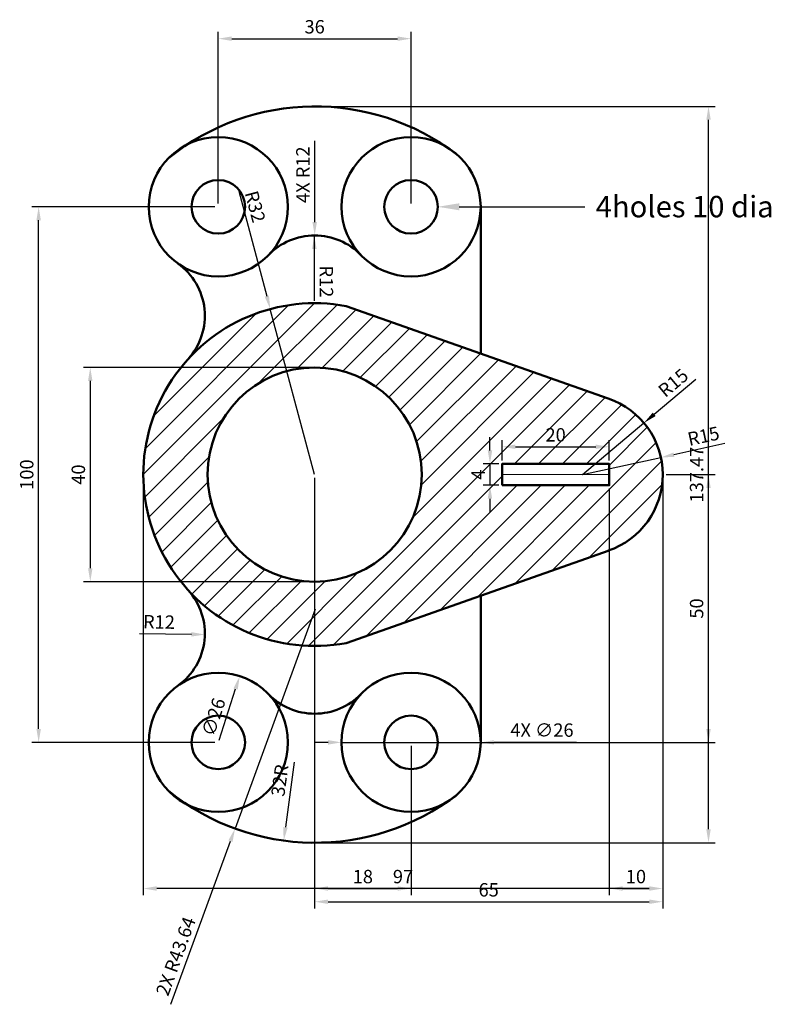
# Model space of a CAD drawing. Units: millimetres. Extents: x 3469 to 3609, y 1274 to 1457.
import ezdxf
from ezdxf import colors
from ezdxf.entities.mleader import LeaderData, LeaderLine
from ezdxf.math import Vec2, Vec3

# ---------------------------------------------------------------- set-up
doc = ezdxf.new("R2010")
doc.units = ezdxf.units.MM
doc.linetypes.add('CENTER', pattern=[50.8, 31.75, -6.35, 6.35, -6.35])
for name, color, linetype, lineweight in [('M-CNTR', 4, 'CENTER', 18), ('M-DIMS', 2, 'Continuous', 25), ('M-HATC', 8, 'Continuous', 18), ('M-OUTL', 7, 'Continuous', 50), ('M-TEXT', 7, 'Continuous', 25)]:
    doc.layers.add(name, color=color, linetype=linetype, lineweight=lineweight)
doc.styles.get("Standard").update_dxf_attribs({"font": 'arial.ttf'})
doc.dimstyles.new('ISO-25', dxfattribs={"dimtxt": 2.5, "dimasz": 2.5, "dimexe": 1.25, "dimexo": 0.625, "dimtad": 1, "dimtxsty": 'Standard', "dimcen": 2.5, "dimadec": 0, "dimazin": 0, "dimtfac": 1, "dimtmove": 0, "dimatfit": 3, "dimfxl": 1, "dimarcsym": 0})

# ---------------------------------------------------------------- blocks, each defined once
blk = doc.blocks.new('*D1')
at = {"layer": 'Defpoints', "color": 0, "transparency": 16777216}
for p in [(3541.88, 1453.9), (3505.88, 1422.51), (3541.88, 1422.51)]:
    blk.add_point(p, dxfattribs=at)
at = {"layer": 'M-DIMS', "color": 0, "lineweight": -2, "transparency": 16777216}
for p, q in [((3505.88, 1423.14), (3505.88, 1455.15)), ((3541.88, 1423.14), (3541.88, 1455.15)), ((3508.38, 1453.9), (3539.38, 1453.9))]:
    blk.add_line(p, q, dxfattribs=at)
at = {"layer": 'M-DIMS', "color": 0, "transparency": 16777216}
for points in [[(3508.38, 1454.32), (3508.38, 1453.49), (3505.88, 1453.9)], [(3539.38, 1454.32), (3539.38, 1453.49), (3541.88, 1453.9)]]:
    blk.add_solid(points, dxfattribs=at)
at = {"layer": 'M-DIMS', "color": 0, "transparency": 16777216, "insert": (3523.88, 1455.8), "char_height": 2.5, "attachment_point": 5}
blk.add_mtext('36', dxfattribs=at)
blk = doc.blocks.new('*D2')
at = {"layer": 'Defpoints', "color": 0, "transparency": 16777216}
for p in [(3523.88, 1372.51), (3588.88, 1372.51), (3588.88, 1292.76)]:
    blk.add_point(p, dxfattribs=at)
at = {"layer": 'M-DIMS', "color": 0, "lineweight": -2, "transparency": 16777216}
for p, q in [((3523.88, 1371.89), (3523.88, 1291.51)), ((3588.88, 1371.89), (3588.88, 1291.51)), ((3526.38, 1292.76), (3586.38, 1292.76))]:
    blk.add_line(p, q, dxfattribs=at)
at = {"layer": 'M-DIMS', "color": 0, "transparency": 16777216}
for points in [[(3526.38, 1293.17), (3526.38, 1292.34), (3523.88, 1292.76)], [(3586.38, 1293.17), (3586.38, 1292.34), (3588.88, 1292.76)]]:
    blk.add_solid(points, dxfattribs=at)
at = {"layer": 'M-DIMS', "color": 0, "transparency": 16777216, "insert": (3556.38, 1294.66), "char_height": 2.5, "attachment_point": 5}
blk.add_mtext('65', dxfattribs=at)
blk = doc.blocks.new('*D3')
at = {"layer": 'Defpoints', "color": 0, "transparency": 16777216}
for p in [(3472.33, 1422.51), (3505.88, 1422.51), (3505.88, 1322.51)]:
    blk.add_point(p, dxfattribs=at)
at = {"layer": 'M-DIMS', "color": 0, "lineweight": -2, "transparency": 16777216}
for p, q in [((3505.26, 1422.51), (3471.08, 1422.51)), ((3472.33, 1325.01), (3472.33, 1420.01)), ((3505.26, 1322.51), (3471.08, 1322.51))]:
    blk.add_line(p, q, dxfattribs=at)
at = {"layer": 'M-DIMS', "color": 0, "transparency": 16777216}
for points in [[(3471.92, 1420.01), (3472.75, 1420.01), (3472.33, 1422.51)], [(3471.92, 1325.01), (3472.75, 1325.01), (3472.33, 1322.51)]]:
    blk.add_solid(points, dxfattribs=at)
at = {"layer": 'M-DIMS', "color": 0, "transparency": 16777216, "insert": (3470.43, 1372.51), "char_height": 2.5, "attachment_point": 5, "rotation": 90}
blk.add_mtext('100', dxfattribs=at)
blk = doc.blocks.new('*D4')
at = {"layer": 'Defpoints', "color": 0, "transparency": 16777216}
for p in [(3523.88, 1392.51), (3481.97, 1352.51), (3523.88, 1352.51)]:
    blk.add_point(p, dxfattribs=at)
at = {"layer": 'M-DIMS', "color": 0, "lineweight": -2, "transparency": 16777216}
for p, q in [((3523.26, 1392.51), (3480.72, 1392.51)), ((3481.97, 1390.01), (3481.97, 1355.01)), ((3523.26, 1352.51), (3480.72, 1352.51))]:
    blk.add_line(p, q, dxfattribs=at)
at = {"layer": 'M-DIMS', "color": 0, "transparency": 16777216}
for points in [[(3481.56, 1390.01), (3482.39, 1390.01), (3481.97, 1392.51)], [(3481.56, 1355.01), (3482.39, 1355.01), (3481.97, 1352.51)]]:
    blk.add_solid(points, dxfattribs=at)
at = {"layer": 'M-DIMS', "color": 0, "transparency": 16777216, "insert": (3480.07, 1372.51), "char_height": 2.5, "attachment_point": 5, "rotation": 90}
blk.add_mtext('40', dxfattribs=at)
blk = doc.blocks.new('*D5')
at = {"layer": 'Defpoints', "color": 0, "transparency": 16777216}
for p in [(3578.88, 1377.7), (3558.88, 1374.51), (3578.88, 1374.51)]:
    blk.add_point(p, dxfattribs=at)
at = {"layer": 'M-DIMS', "color": 0, "lineweight": -2, "transparency": 16777216}
for p, q in [((3558.88, 1375.14), (3558.88, 1378.95)), ((3578.88, 1375.14), (3578.88, 1378.95)), ((3561.38, 1377.7), (3576.38, 1377.7))]:
    blk.add_line(p, q, dxfattribs=at)
at = {"layer": 'M-DIMS', "color": 0, "transparency": 16777216}
for points in [[(3561.38, 1378.12), (3561.38, 1377.29), (3558.88, 1377.7)], [(3576.38, 1378.12), (3576.38, 1377.29), (3578.88, 1377.7)]]:
    blk.add_solid(points, dxfattribs=at)
at = {"layer": 'M-DIMS', "color": 0, "transparency": 16777216, "insert": (3568.88, 1379.61), "char_height": 2.5, "attachment_point": 5}
blk.add_mtext('20', dxfattribs=at)
blk = doc.blocks.new('*D6')
at = {"layer": 'Defpoints', "color": 0, "transparency": 16777216}
for p in [(3558.88, 1374.51), (3556.62, 1370.51), (3558.88, 1370.51)]:
    blk.add_point(p, dxfattribs=at)
at = {"layer": 'M-DIMS', "color": 0, "lineweight": -2, "transparency": 16777216}
for p, q in [((3556.62, 1377.01), (3556.62, 1379.51)), ((3558.26, 1374.51), (3555.37, 1374.51)), ((3556.62, 1374.51), (3556.62, 1370.51)), ((3558.26, 1370.51), (3555.37, 1370.51)), ((3556.62, 1368.01), (3556.62, 1365.51))]:
    blk.add_line(p, q, dxfattribs=at)
at = {"layer": 'M-DIMS', "color": 0, "transparency": 16777216}
for points in [[(3556.2, 1377.01), (3557.03, 1377.01), (3556.62, 1374.51)], [(3556.2, 1368.01), (3557.03, 1368.01), (3556.62, 1370.51)]]:
    blk.add_solid(points, dxfattribs=at)
at = {"layer": 'M-DIMS', "color": 0, "transparency": 16777216, "insert": (3554.74, 1372.51), "char_height": 2.5, "attachment_point": 5, "rotation": 90}
blk.add_mtext('4', dxfattribs=at)
blk = doc.blocks.new('*D7')
at = {"layer": 'Defpoints', "color": 0, "transparency": 16777216}
for p in [(3509.89, 1334.88), (3501.88, 1310.14)]:
    blk.add_point(p, dxfattribs=at)
at = {"layer": 'M-DIMS', "color": 0, "lineweight": -2, "transparency": 16777216}
blk.add_line((3506.02, 1322.94), (3509.12, 1332.5), dxfattribs=at)
at = {"layer": 'M-DIMS', "color": 0, "transparency": 16777216}
blk.add_solid([(3508.72, 1332.63), (3509.51, 1332.37), (3509.89, 1334.88)], dxfattribs=at)
at = {"layer": 'M-DIMS', "color": 0, "transparency": 16777216, "insert": (3505.31, 1327.14), "char_height": 2.5, "attachment_point": 5, "rotation": 72.0514}
blk.add_mtext('∅26', dxfattribs=at)
blk = doc.blocks.new('*D8')
at = {"layer": 'Defpoints', "color": 0, "transparency": 16777216}
for p in [(3523.96, 1347.41), (3518.09, 1304.17)]:
    blk.add_point(p, dxfattribs=at)
at = {"layer": 'M-DIMS', "color": 0, "lineweight": -2, "transparency": 16777216}
blk.add_line((3520.08, 1318.8), (3518.43, 1306.65), dxfattribs=at)
at = {"layer": 'M-DIMS', "color": 0, "transparency": 16777216}
blk.add_solid([(3518.01, 1306.7), (3518.84, 1306.59), (3518.09, 1304.17)], dxfattribs=at)
at = {"layer": 'M-DIMS', "color": 0, "transparency": 16777216, "insert": (3517.69, 1315.36), "char_height": 2.5, "attachment_point": 5, "rotation": 82.2703}
blk.add_mtext('32R', dxfattribs=at)
blk = doc.blocks.new('*D9')
at = {"layer": 'Defpoints', "color": 0, "transparency": 16777216}
for p in [(3588.54, 1375.7), (3573.88, 1372.51)]:
    blk.add_point(p, dxfattribs=at)
at = {"layer": 'M-DIMS', "color": 0, "lineweight": -2, "transparency": 16777216}
for p, q in [((3600.5, 1378.3), (3590.98, 1376.23)), ((3573.88, 1372.51), (3588.54, 1375.7))]:
    blk.add_line(p, q, dxfattribs=at)
at = {"layer": 'M-DIMS', "color": 0, "transparency": 16777216}
blk.add_solid([(3590.89, 1376.64), (3591.07, 1375.82), (3588.54, 1375.7)], dxfattribs=at)
at = {"layer": 'M-DIMS', "color": 0, "transparency": 16777216, "insert": (3596.56, 1379.39), "char_height": 2.5, "attachment_point": 5, "rotation": 12.2647}
blk.add_mtext('R15', dxfattribs=at)
blk = doc.blocks.new('*D10')
at = {"layer": 'Defpoints', "color": 0, "transparency": 16777216}
for p in [(3491.37, 1342.87), (3503.37, 1342.64)]:
    blk.add_point(p, dxfattribs=at)
at = {"layer": 'M-DIMS', "color": 0, "lineweight": -2, "transparency": 16777216}
blk.add_line((3491.17, 1342.87), (3500.87, 1342.69), dxfattribs=at)
at = {"layer": 'M-DIMS', "color": 0, "transparency": 16777216}
blk.add_solid([(3500.87, 1343.1), (3500.86, 1342.27), (3503.37, 1342.64)], dxfattribs=at)
at = {"layer": 'M-DIMS', "color": 0, "transparency": 16777216, "insert": (3494.8, 1344.68), "char_height": 2.5, "attachment_point": 5, "rotation": 358.9032}
blk.add_mtext('R12', dxfattribs=at)
blk = doc.blocks.new('*D11')
at = {"layer": 'Defpoints', "color": 0, "transparency": 16777216}
for p in [(3523.81, 1417.16), (3523.88, 1405.16)]:
    blk.add_point(p, dxfattribs=at)
at = {"layer": 'M-DIMS', "color": 0, "lineweight": -2, "transparency": 16777216}
blk.add_line((3523.88, 1404.96), (3523.83, 1414.66), dxfattribs=at)
at = {"layer": 'M-DIMS', "color": 0, "transparency": 16777216}
blk.add_solid([(3524.24, 1414.66), (3523.41, 1414.66), (3523.81, 1417.16)], dxfattribs=at)
at = {"layer": 'M-DIMS', "color": 0, "transparency": 16777216, "insert": (3525.74, 1408.57), "char_height": 2.5, "attachment_point": 5, "rotation": 270.331}
blk.add_mtext('R12', dxfattribs=at)
blk = doc.blocks.new('MOUNT-HOLE-D10-BOSS-D26')
for radius in [13, 5]:
    blk.add_circle((0, 0), radius)
blk = doc.blocks.new('*D13')
at = {"layer": 'Defpoints', "color": 0, "transparency": 16777216}
for p in [(3523.38, 1441.25), (3597.43, 1441.25), (3523.38, 1303.78)]:
    blk.add_point(p, dxfattribs=at)
at = {"layer": 'M-DIMS', "color": 0, "lineweight": -2, "transparency": 16777216}
for p, q in [((3524.01, 1441.25), (3598.68, 1441.25)), ((3597.43, 1306.28), (3597.43, 1438.75)), ((3524.01, 1303.78), (3598.68, 1303.78))]:
    blk.add_line(p, q, dxfattribs=at)
at = {"layer": 'M-DIMS', "color": 0, "transparency": 16777216}
for points in [[(3597.02, 1438.75), (3597.85, 1438.75), (3597.43, 1441.25)], [(3597.02, 1306.28), (3597.85, 1306.28), (3597.43, 1303.78)]]:
    blk.add_solid(points, dxfattribs=at)
at = {"layer": 'M-DIMS', "color": 0, "transparency": 16777216, "insert": (3595.53, 1372.51), "char_height": 2.5, "attachment_point": 5, "rotation": 90}
blk.add_mtext('137.47', dxfattribs=at)
blk = doc.blocks.new('*D14')
at = {"layer": 'Defpoints', "color": 0, "transparency": 16777216}
for p in [(3491.88, 1372.51), (3588.88, 1372.51), (3491.88, 1295.23)]:
    blk.add_point(p, dxfattribs=at)
at = {"layer": 'M-DIMS', "color": 0, "lineweight": -2, "transparency": 16777216}
for p, q in [((3491.88, 1371.89), (3491.88, 1293.98)), ((3588.88, 1371.89), (3588.88, 1293.98)), ((3586.38, 1295.23), (3494.38, 1295.23))]:
    blk.add_line(p, q, dxfattribs=at)
at = {"layer": 'M-DIMS', "color": 0, "transparency": 16777216}
for points in [[(3494.38, 1295.64), (3494.38, 1294.81), (3491.88, 1295.23)], [(3586.38, 1295.64), (3586.38, 1294.81), (3588.88, 1295.23)]]:
    blk.add_solid(points, dxfattribs=at)
at = {"layer": 'M-DIMS', "color": 0, "transparency": 16777216, "insert": (3540.38, 1297.13), "char_height": 2.5, "attachment_point": 5}
blk.add_mtext('97', dxfattribs=at)
blk = doc.blocks.new('*D15')
at = {"layer": 'Defpoints', "color": 0, "transparency": 16777216}
for p in [(3523.88, 1352.51), (3541.88, 1322.51), (3541.88, 1295.23)]:
    blk.add_point(p, dxfattribs=at)
at = {"layer": 'M-DIMS', "color": 0, "lineweight": -2, "transparency": 16777216}
for p, q in [((3523.88, 1351.89), (3523.88, 1293.98)), ((3541.88, 1321.89), (3541.88, 1293.98)), ((3526.38, 1295.23), (3539.38, 1295.23))]:
    blk.add_line(p, q, dxfattribs=at)
at = {"layer": 'M-DIMS', "color": 0, "transparency": 16777216}
for points in [[(3526.38, 1295.64), (3526.38, 1294.81), (3523.88, 1295.23)], [(3539.38, 1295.64), (3539.38, 1294.81), (3541.88, 1295.23)]]:
    blk.add_solid(points, dxfattribs=at)
at = {"layer": 'M-DIMS', "color": 0, "transparency": 16777216, "insert": (3532.88, 1297.13), "char_height": 2.5, "attachment_point": 5}
blk.add_mtext('18', dxfattribs=at)
blk = doc.blocks.new('*D16')
at = {"layer": 'Defpoints', "color": 0, "transparency": 16777216}
for p in [(3588.88, 1372.51), (3597.43, 1372.51), (3541.88, 1322.51)]:
    blk.add_point(p, dxfattribs=at)
at = {"layer": 'M-DIMS', "color": 0, "lineweight": -2, "transparency": 16777216}
for p, q in [((3589.51, 1372.51), (3598.68, 1372.51)), ((3597.43, 1325.01), (3597.43, 1370.01)), ((3542.51, 1322.51), (3598.68, 1322.51))]:
    blk.add_line(p, q, dxfattribs=at)
at = {"layer": 'M-DIMS', "color": 0, "transparency": 16777216}
for points in [[(3597.02, 1370.01), (3597.85, 1370.01), (3597.43, 1372.51)], [(3597.02, 1325.01), (3597.85, 1325.01), (3597.43, 1322.51)]]:
    blk.add_solid(points, dxfattribs=at)
at = {"layer": 'M-DIMS', "color": 0, "transparency": 16777216, "insert": (3595.53, 1347.51), "char_height": 2.5, "attachment_point": 5, "rotation": 90}
blk.add_mtext('50', dxfattribs=at)
blk = doc.blocks.new('*D17')
at = {"layer": 'Defpoints', "color": 0, "transparency": 16777216}
for p in [(3588.88, 1372.51), (3578.88, 1370.51), (3588.88, 1295.23)]:
    blk.add_point(p, dxfattribs=at)
at = {"layer": 'M-DIMS', "color": 0, "lineweight": -2, "transparency": 16777216}
for p, q in [((3588.88, 1371.89), (3588.88, 1293.98)), ((3578.88, 1369.89), (3578.88, 1293.98)), ((3581.38, 1295.23), (3586.38, 1295.23))]:
    blk.add_line(p, q, dxfattribs=at)
at = {"layer": 'M-DIMS', "color": 0, "transparency": 16777216}
for points in [[(3581.38, 1295.64), (3581.38, 1294.81), (3578.88, 1295.23)], [(3586.38, 1295.64), (3586.38, 1294.81), (3588.88, 1295.23)]]:
    blk.add_solid(points, dxfattribs=at)
at = {"layer": 'M-DIMS', "color": 0, "transparency": 16777216, "insert": (3583.88, 1297.13), "char_height": 2.5, "attachment_point": 5}
blk.add_mtext('10', dxfattribs=at)
blk = doc.blocks.new('*D18')
at = {"layer": 'Defpoints', "color": 0, "transparency": 16777216}
for p in [(3523.96, 1347.41), (3509.01, 1306.42)]:
    blk.add_point(p, dxfattribs=at)
at = {"layer": 'M-DIMS', "color": 0, "lineweight": -2, "transparency": 16777216}
for p, q in [((3523.96, 1347.41), (3509.01, 1306.42)), ((3497.04, 1273.61), (3508.15, 1304.07))]:
    blk.add_line(p, q, dxfattribs=at)
at = {"layer": 'M-DIMS', "color": 0, "transparency": 16777216}
blk.add_solid([(3507.76, 1304.21), (3508.54, 1303.92), (3509.01, 1306.42)], dxfattribs=at)
at = {"layer": 'M-DIMS', "color": 0, "transparency": 16777216, "insert": (3498.25, 1282.47), "char_height": 2.5, "attachment_point": 5, "rotation": 69.9596}
blk.add_mtext('2X R43.64', dxfattribs=at)
blk = doc.blocks.new('*D19')
at = {"layer": 'Defpoints', "color": 0, "transparency": 16777216}
for p in [(3515.59, 1403.42), (3523.88, 1372.51)]:
    blk.add_point(p, dxfattribs=at)
at = {"layer": 'M-DIMS', "color": 0, "lineweight": -2, "transparency": 16777216}
for p, q in [((3509.69, 1425.44), (3514.95, 1405.83)), ((3523.88, 1372.51), (3515.59, 1403.42))]:
    blk.add_line(p, q, dxfattribs=at)
at = {"layer": 'M-DIMS', "color": 0, "transparency": 16777216}
blk.add_solid([(3515.35, 1405.94), (3514.54, 1405.73), (3515.59, 1403.42)], dxfattribs=at)
at = {"layer": 'M-DIMS', "color": 0, "transparency": 16777216, "insert": (3512.46, 1422.46), "char_height": 2.5, "attachment_point": 5, "rotation": 285.0091}
blk.add_mtext('R32', dxfattribs=at)
blk = doc.blocks.new('*D20')
at = {"layer": 'Defpoints', "color": 0, "transparency": 16777216}
for p in [(3585.37, 1382.15), (3573.88, 1372.51)]:
    blk.add_point(p, dxfattribs=at)
at = {"layer": 'M-DIMS', "color": 0, "lineweight": -2, "transparency": 16777216}
for p, q in [((3595.04, 1390.26), (3587.29, 1383.76)), ((3573.88, 1372.51), (3585.37, 1382.15))]:
    blk.add_line(p, q, dxfattribs=at)
at = {"layer": 'M-DIMS', "color": 0, "transparency": 16777216}
blk.add_solid([(3587.02, 1384.08), (3587.56, 1383.44), (3585.37, 1382.15)], dxfattribs=at)
at = {"layer": 'M-DIMS', "color": 0, "transparency": 16777216, "insert": (3591.05, 1389.39), "char_height": 2.5, "attachment_point": 5, "rotation": 39.9953}
blk.add_mtext('R15', dxfattribs=at)
blk = doc.blocks.new('*D21')
at = {"layer": 'Defpoints', "color": 0, "transparency": 16777216}
for p in [(3523.88, 1417.16), (3523.88, 1405.16)]:
    blk.add_point(p, dxfattribs=at)
at = {"layer": 'M-DIMS', "color": 0, "lineweight": -2, "transparency": 16777216}
for p, q in [((3523.88, 1434.83), (3523.88, 1419.66)), ((3523.88, 1405.16), (3523.88, 1417.16))]:
    blk.add_line(p, q, dxfattribs=at)
at = {"layer": 'M-DIMS', "color": 0, "transparency": 16777216}
blk.add_solid([(3523.47, 1419.66), (3524.3, 1419.66), (3523.88, 1417.16)], dxfattribs=at)
at = {"layer": 'M-DIMS', "color": 0, "transparency": 16777216, "insert": (3522, 1428.5), "char_height": 2.5, "attachment_point": 5, "rotation": 89.9987}
blk.add_mtext('4X R12', dxfattribs=at)
blk = doc.blocks.new('*D22')
at = {"layer": 'Defpoints', "color": 0, "transparency": 16777216}
for p in [(3528.88, 1322.51), (3554.88, 1322.51)]:
    blk.add_point(p, dxfattribs=at)
at = {"layer": 'M-DIMS', "color": 0, "lineweight": -2, "transparency": 16777216}
for p, q in [((3526.38, 1322.51), (3523.88, 1322.51)), ((3528.88, 1322.51), (3554.88, 1322.51)), ((3572.77, 1322.51), (3557.38, 1322.51))]:
    blk.add_line(p, q, dxfattribs=at)
at = {"layer": 'M-DIMS', "color": 0, "transparency": 16777216}
for points in [[(3526.38, 1322.93), (3526.38, 1322.09), (3528.88, 1322.51)], [(3557.38, 1322.93), (3557.38, 1322.1), (3554.88, 1322.51)]]:
    blk.add_solid(points, dxfattribs=at)
at = {"layer": 'M-DIMS', "color": 0, "transparency": 16777216, "insert": (3566.33, 1324.48), "char_height": 2.5, "attachment_point": 5, "rotation": 0.0009}
blk.add_mtext('4X ∅26', dxfattribs=at)

msp = doc.modelspace()

# ---------------------------------------------------------------- hatches: boundary and pattern name
at = {"layer": 'M-HATC'}
h = msp.add_hatch(dxfattribs=at)
h.set_pattern_fill('ANSI31', color=256)
h.paths.add_polyline_path([(3578.705, 1386.715), (3529.782, 1403.963, 1.2050619), (3529.782, 1341.061), (3578.869, 1358.365, 0.7121472)])
h.paths.add_polyline_path([(3543.882, 1372.512, -1), (3503.882, 1372.512, -1)], flags=16)
h.paths.add_polyline_path([(3558.882, 1374.512), (3578.882, 1374.512), (3578.882, 1370.512), (3558.882, 1370.512), (3558.882, 1372.512)], flags=16)

# ---------------------------------------------------------------- linework, layer by layer
at = {"layer": 'M-CNTR'}
msp.add_line((3558.882, 1372.512), (3578.882, 1372.512), dxfattribs=at)
at = {"layer": 'M-OUTL'}
for p, q in [((3554.882, 1422.512), (3554.882, 1395.097)), ((3529.782, 1341.061), (3578.869, 1358.365)), ((3554.882, 1322.512), (3554.882, 1349.9))]:
    msp.add_line(p, q, dxfattribs=at)
msp.add_lwpolyline([(3578.705, 1358.308, 0.7165249), (3578.705, 1386.715), (3529.782, 1403.963)], format="xyb", dxfattribs=at)
msp.add_lwpolyline([(3558.882, 1370.512), (3578.882, 1370.512), (3578.882, 1374.512), (3558.882, 1374.512), (3558.882, 1372.512)], close=True, dxfattribs=at)
msp.add_circle((3523.882, 1372.512), 20, dxfattribs=at)
for centre, radius, start, end in [((3523.96, 1397.612), 43.639, 52.64744, 128.87292), ((3523.882, 1405.162), 12, 43.94552, 136.05448), ((3491.367, 1402.157), 12, 317.64315, 54.50902), ((3523.882, 1372.512), 32, 79.37401, 280.62599), ((3491.367, 1342.867), 12, 305.49098, 42.35685), ((3523.882, 1339.861), 12, 223.94552, 316.05448), ((3523.96, 1347.412), 43.639, 231.12708, 307.35256)]:
    msp.add_arc(centre, radius, start, end, dxfattribs=at)

# ---------------------------------------------------------------- block references
for p in [(3505.882, 1422.512), (3541.882, 1422.512), (3505.882, 1322.512), (3541.882, 1322.512)]:
    msp.add_blockref('MOUNT-HOLE-D10-BOSS-D26', p, dxfattribs=at)

# ---------------------------------------------------------------- dimensions: what is measured, and where the dimension line sits
at = {"layer": 'M-DIMS'}
for base, p1, p2, override, picture, middle in [((3541.882, 1453.902), (3505.882, 1422.512), (3541.882, 1422.512), {"dimclrd": 0, "dimclre": 0, "dimclrt": 0}, '*D1', (3523.882, 1455.805)), ((3578.882, 1377.704), (3558.882, 1374.512), (3578.882, 1374.512), {"dimclrd": 0, "dimclre": 0, "dimclrt": 0}, '*D5', (3568.882, 1379.605)), ((3491.882, 1295.227), (3588.882, 1372.512), (3491.882, 1372.512), {"dimdec": 0, "dimlfac": 1, "dimrnd": 0, "dimzin": 0, "dimdsep": 46, "dimlunit": 2}, '*D14', (3540.382, 1297.129)), ((3588.882, 1292.757), (3523.882, 1372.512), (3588.882, 1372.512), {"dimclrd": 0, "dimclre": 0, "dimclrt": 0}, '*D2', (3556.382, 1294.659)), ((3588.882, 1295.227), (3578.882, 1370.512), (3588.882, 1372.512), {"dimdec": 0, "dimlfac": 1, "dimrnd": 0, "dimzin": 0, "dimdsep": 46, "dimlunit": 2}, '*D17', (3583.882, 1297.129)), ((3541.882, 1295.227), (3523.882, 1352.512), (3541.882, 1322.512), {"dimdec": 0, "dimlfac": 1, "dimrnd": 0, "dimzin": 0, "dimdsep": 46, "dimlunit": 2}, '*D15', (3532.882, 1297.129))]:
    dim = msp.add_linear_dim(base=base, p1=p1, p2=p2, dimstyle='ISO-25', override=override, dxfattribs=at)
    dim.commit()
    dim.dimension.update_dxf_attribs({"geometry": picture, "text_midpoint": middle})
for base, p1, p2, override, picture, middle in [((3597.432, 1441.246), (3523.381, 1303.777), (3523.381, 1441.246), {"dimdec": 2, "dimlfac": 1, "dimrnd": 0, "dimzin": 0, "dimdsep": 46, "dimlunit": 2}, '*D13', (3595.529, 1372.512)), ((3472.334, 1422.512), (3505.882, 1322.512), (3505.882, 1422.512), {"dimclrd": 0, "dimclre": 0, "dimclrt": 0}, '*D3', (3470.432, 1372.512)), ((3481.973, 1352.512), (3523.882, 1392.512), (3523.882, 1352.512), {"dimclrd": 0, "dimclre": 0, "dimclrt": 0}, '*D4', (3480.072, 1372.512)), ((3556.615, 1370.512), (3558.882, 1374.512), (3558.882, 1370.512), {"dimclrd": 0, "dimclre": 0, "dimclrt": 0}, '*D6', (3554.74, 1372.512)), ((3597.432, 1372.512), (3541.882, 1322.512), (3588.882, 1372.512), {"dimdec": 0, "dimlfac": 1, "dimrnd": 0, "dimzin": 0, "dimdsep": 46, "dimlunit": 2}, '*D16', (3595.53, 1347.512))]:
    dim = msp.add_linear_dim(base=base, p1=p1, p2=p2, angle=90, dimstyle='ISO-25', override=override, dxfattribs=at)
    dim.commit()
    dim.dimension.update_dxf_attribs({"geometry": picture, "text_midpoint": middle})
dim = msp.add_radius_dim(center=(3523.882, 1405.162), mpoint=(3523.882, 1417.162), text='4X <>', dimstyle='ISO-25', override={"dimdec": 0, "dimlfac": 1, "dimrnd": 0, "dimzin": 0, "dimdsep": 46, "dimlunit": 2}, dxfattribs=at)
dim.commit()
dim.dimension.update_dxf_attribs({"geometry": '*D21', "text_midpoint": (3522.001, 1428.498)})
for center, mpoint, override, picture, middle in [((3523.882, 1372.512), (3515.595, 1403.42), {"dimdec": 0, "dimlfac": 1, "dimrnd": 0, "dimzin": 0, "dimdsep": 46, "dimlunit": 2}, '*D19', (3510.622, 1421.965)), ((3523.882, 1405.162), (3523.812, 1417.162), {"dimclrd": 0, "dimclre": 0, "dimclrt": 0}, '*D11', (3523.862, 1408.563)), ((3573.882, 1372.512), (3585.373, 1382.153), {"dimdec": 0, "dimlfac": 1, "dimrnd": 0, "dimzin": 0, "dimdsep": 46, "dimlunit": 2}, '*D20', (3592.268, 1387.937)), ((3491.367, 1342.867), (3503.365, 1342.637), {"dimclrd": 0, "dimclre": 0, "dimclrt": 0}, '*D10', (3494.768, 1342.802))]:
    dim = msp.add_radius_dim(center=center, mpoint=mpoint, dimstyle='ISO-25', override=override, dxfattribs=at)
    dim.commit()
    dim.dimension.update_dxf_attribs({"geometry": picture, "text_midpoint": middle, "dimtype": 164})
dim = msp.add_radius_dim(center=(3573.882, 1372.512), mpoint=(3588.539, 1375.698), dimstyle='ISO-25', override={"dimclrd": 0, "dimclre": 0, "dimclrt": 0}, dxfattribs=at)
dim.commit()
dim.dimension.update_dxf_attribs({"geometry": '*D9', "text_midpoint": (3596.56, 1379.388)})
for mpoint, text, override, picture, middle in [((3509.006, 1306.416), '2X <>', {"dimdec": 2, "dimlfac": 1, "dimrnd": 0, "dimzin": 0, "dimdsep": 46, "dimlunit": 2}, '*D18', (3500.033, 1281.818)), ((3518.091, 1304.17), '32R', {"dimclrd": 0, "dimclre": 0, "dimclrt": 0}, '*D8', (3519.575, 1315.104))]:
    dim = msp.add_radius_dim(center=(3523.96, 1347.412), mpoint=mpoint, text=text, dimstyle='ISO-25', override=override, dxfattribs=at)
    dim.commit()
    dim.dimension.update_dxf_attribs({"geometry": picture, "text_midpoint": middle, "dimtype": 164})
dim = msp.add_diameter_dim_2p(p1=(3501.876, 1310.144), p2=(3509.888, 1334.879), dimstyle='ISO-25', override={"dimclrd": 0, "dimclre": 0, "dimclrt": 0}, dxfattribs=at)
dim.commit()
dim.dimension.update_dxf_attribs({"geometry": '*D7', "text_midpoint": (3507.184, 1326.531), "dimtype": 163})
dim = msp.add_diameter_dim_2p(p1=(3528.882, 1322.512), p2=(3554.882, 1322.512), text='4X <>', dimstyle='ISO-25', override={"dimdec": 0, "dimlfac": 1, "dimrnd": 0, "dimzin": 0, "dimdsep": 46, "dimlunit": 2}, dxfattribs=at)
dim.commit()
dim.dimension.update_dxf_attribs({"geometry": '*D22', "text_midpoint": (3566.326, 1322.512), "dimtype": 163})

# ---------------------------------------------------------------- leaders
at = {"layer": 'M-TEXT'}
ml = msp.add_multileader_mtext('Standard', dxfattribs=at)
ml.set_content('4holes 10 dia', color=256)
ml.set_leader_properties()
ml.build(insert=Vec2(0, 0))
ctx = ml.context
ctx.base_point, ctx.plane_origin = Vec3(3574.364, 1422.512), Vec3(3546.882, 1422.512)
notes = []
notes.append((ctx, [(0, (1, 1, 0), (3566.364, 1422.512), (1, 0), 8, [(0, [(3546.882, 1422.512)], 0, [])])]))
ctx.mtext.insert, ctx.mtext.flow_direction = Vec3(3576.364, 1424.546), 5
for ctx, leaders in notes:
    for number, flags, end, landing, length, lines in leaders:
        leader = LeaderData()
        leader.index, (leader.has_last_leader_line, leader.has_dogleg_vector, leader.attachment_direction) = number, flags
        leader.last_leader_point, leader.dogleg_vector, leader.dogleg_length = Vec3(end), Vec3(landing), length
        for number, points, colour, breaks in lines:
            line = LeaderLine()
            line.index, line.vertices, line.color, line.breaks = number, Vec3.list(points), colors.encode_raw_color(colour), breaks
            leader.lines.append(line)
        ctx.leaders.append(leader)

doc.saveas('drawing.dxf')
